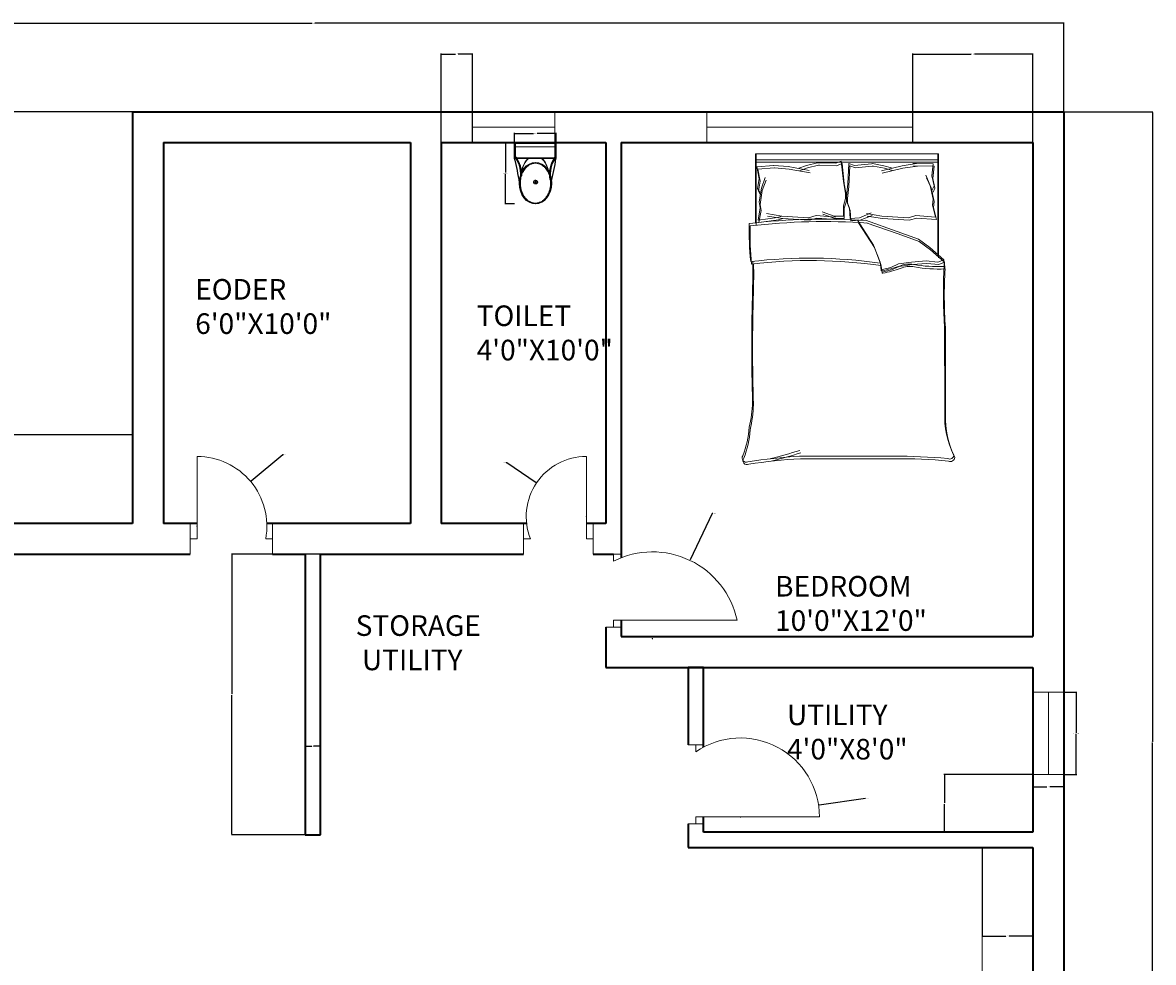
# Model space of a CAD drawing. Units: inches. Extents: x 2067 to 3463, y 1605 to 2723.
# Tile 5 of 10: x 2403 to 2733, y 1910 to 2184. Entities that reach past the tile are written whole.
import ezdxf

# ---------------------------------------------------------------- set-up
doc = ezdxf.new("R2010")
doc.units = ezdxf.units.IN
for name, color, linetype, lineweight in [('A-ANNO-DIMS', 2, 'Continuous', 18), ('A-AREA-IDEN', 7, 'Continuous', 18), ('A-DOOR', 3, 'Continuous', 18), ('A-FLOR-CASE', 8, 'Continuous', 18), ('A-FLOR-FIXT', 8, 'Continuous', 18), ('A-FURN', 8, 'Continuous', 13), ('A-GLAZ', 4, 'Continuous', 18), ('A-WALL', 7, 'Continuous', 35)]:
    doc.layers.add(name, color=color, linetype=linetype, lineweight=lineweight)
doc.styles.get("Standard").update_dxf_attribs({"font": 'arial.ttf'})
doc.dimstyles.get("Standard").update_dxf_attribs({"dimtxt": 0.18, "dimasz": 0.18, "dimexe": 0.18, "dimexo": 0.0625, "dimgap": 0.09, "dimtad": 0, "dimtih": 1, "dimtoh": 1, "dimdec": 4, "dimzin": 0, "dimdsep": 46, "dimtxsty": 'Standard', "dimcen": 0.09, "dimadec": 0, "dimazin": 0, "dimtfac": 1, "dimtdec": 4, "dimtofl": 0, "dimtmove": 0, "dimatfit": 3, "dimfxl": 1, "dimtolj": 1, "dimtzin": 0, "dimarcsym": 0})

# ---------------------------------------------------------------- blocks, each defined once
blk = doc.blocks.new('A$C31115884')
for p, q in [((283, 498), (223, 498)), ((258, 466), (258, 523)), ((0, 200), (0, 0)), ((520, 200), (0, 200)), ((10, 190), (10, 10)), ((510, 190), (10, 190)), ((510, 10), (510, 190)), ((520, 0), (520, 200)), ((510, 54), (0, 54)), ((10, 10), (510, 10)), ((0, 0), (520, 0))]:
    blk.add_line(p, q)
blk.add_circle((256, 496), 23.6)
for centre, radius, start, end in [((2778, -205), 2807, 165.4549, 171.7133), ((-295, 403), 365, 324.2091, 9.3499), ((-295, 403), 375, 324.2091, 9.3499), ((806, 403), 365, 170.6501, 215.7909), ((3237, 905), 2807, 188.2867, 194.5451), ((384, 406), 293, 190.2774, 224.1564), ((139, 406), 293, 315.8436, 2.6563), ((806, 403), 375, 179.2036, 215.7909)]:
    blk.add_arc(centre, radius, start, end)
blk.add_ellipse((256, 510), major_axis=(0, -261), ratio=0.772727)
blk.add_open_spline([(256, 259), (263, 259), (270, 260), (288, 262), (299, 265), (320, 273), (330, 278), (350, 291), (360, 299), (378, 316), (386, 326), (402, 347), (409, 358), (421, 383), (427, 395), (436, 422), (440, 436), (445, 465), (447, 480), (448, 509), (448, 524), (445, 553), (443, 568), (436, 596), (432, 610), (422, 636), (416, 649), (402, 672), (395, 683), (379, 703), (370, 712), (351, 728), (341, 735), (321, 746), (310, 751), (289, 757), (278, 759), (256, 761), (245, 761), (223, 757), (212, 754), (191, 746), (181, 741), (161, 728), (151, 720), (133, 703), (125, 693), (110, 672), (103, 660), (90, 636), (85, 623), (76, 596), (72, 582), (67, 553), (66, 538), (64, 509), (65, 494), (68, 465), (70, 450), (77, 422), (81, 408), (91, 382), (97, 370), (111, 346), (118, 335), (135, 316), (144, 307), (162, 291), (172, 284), (193, 273), (203, 269), (225, 262), (236, 260), (250, 259), (253, 259), (256, 259)], degree=3, knots=[0, 0, 0, 0, 0.110105, 0.110105, 0.285049, 0.285049, 0.459994, 0.459994, 0.634938, 0.634938, 0.809882, 0.809882, 0.984827, 0.984827, 1.159771, 1.159771, 1.334715, 1.334715, 1.50966, 1.50966, 1.684604, 1.684604, 1.859549, 1.859549, 2.034493, 2.034493, 2.209437, 2.209437, 2.384382, 2.384382, 2.559326, 2.559326, 2.73427, 2.73427, 2.909215, 2.909215, 3.084159, 3.084159, 3.259103, 3.259103, 3.434048, 3.434048, 3.608992, 3.608992, 3.783936, 3.783936, 3.958881, 3.958881, 4.133825, 4.133825, 4.30877, 4.30877, 4.483714, 4.483714, 4.658658, 4.658658, 4.833603, 4.833603, 5.008547, 5.008547, 5.183491, 5.183491, 5.358436, 5.358436, 5.53338, 5.53338, 5.708324, 5.708324, 5.883269, 5.883269, 6.058213, 6.058213, 6.233158, 6.233158, 6.283185, 6.283185, 6.283185, 6.283185])
blk = doc.blocks.new('BED-DOUBLE')
for p, q in [((3.86, 70.43), (3.86, 90.57)), ((3.86, 90.57), (57.01, 90.57)), ((4.12, 89.85), (4.12, 90.57)), ((4.12, 69.72), (4.12, 89.85)), ((57.01, 90.57), (57.01, 60.97)), ((57.01, 90.57), (57.26, 90.57)), ((57.26, 90.57), (57.26, 89.74)), ((57.26, 89.85), (57.26, 60.26)), ((3.86, 88.86), (57.01, 88.86)), ((4.12, 88.15), (57.26, 88.15)), ((4.33, 86.88), (4.97, 83.34)), ((4.34, 86.85), (9.1, 87.22)), ((4.59, 86.14), (9.35, 86.51)), ((4.59, 86.17), (5.23, 82.63)), ((9.1, 87.22), (9.21, 87.2)), ((9.21, 87.2), (13.46, 86.88)), ((9.35, 86.51), (9.47, 86.49)), ((9.47, 86.49), (13.72, 86.17)), ((13.46, 86.88), (19.57, 85.75)), ((13.72, 86.17), (19.83, 85.04)), ((16.52, 86.4), (18.77, 87.2)), ((16.77, 85.68), (19.02, 86.49)), ((18.77, 87.2), (21.98, 88)), ((19.02, 86.49), (22.24, 87.29)), ((21.98, 88), (22.34, 88)), ((22.24, 87.29), (22.6, 87.29)), ((22.34, 88), (27.29, 87.84)), ((22.6, 87.29), (27.54, 87.13)), ((27.29, 87.84), (28.89, 88.49)), ((27.54, 87.13), (29.15, 87.77)), ((28.89, 88.49), (29.54, 82.54)), ((29.15, 87.77), (29.79, 81.83)), ((31.11, 87.79), (30.84, 81.82)), ((31.36, 87.08), (31.09, 81.11)), ((32.76, 87.25), (31.11, 87.79)), ((33.01, 86.54), (31.36, 87.08)), ((37.68, 87.72), (32.76, 87.25)), ((37.93, 87.01), (33.01, 86.54)), ((38.04, 87.74), (37.68, 87.72)), ((38.29, 87.03), (37.93, 87.01)), ((41.29, 87.14), (38.04, 87.74)), ((41.55, 86.43), (38.29, 87.03)), ((46.61, 87.15), (40.58, 85.65)), ((46.86, 86.44), (40.84, 84.94)), ((43.59, 86.48), (41.29, 87.14)), ((43.85, 85.77), (41.55, 86.43)), ((50.83, 87.74), (46.61, 87.15)), ((51.09, 87.03), (46.86, 86.44)), ((55.73, 87.72), (49.72, 87.83)), ((49.72, 87.83), (50.83, 87.74)), ((55.98, 87.01), (49.97, 87.12)), ((49.97, 87.12), (51.09, 87.03)), ((55.73, 87.72), (55.3, 84.15)), ((55.98, 87.01), (55.56, 83.44)), ((4.97, 83.34), (4.49, 80.45)), ((5.23, 82.63), (4.75, 79.74)), ((5.62, 80.61), (6.74, 83.66)), ((5.87, 79.9), (7, 82.95)), ((29.54, 82.54), (30.18, 79)), ((54.83, 81.38), (53.52, 84.36)), ((55.09, 80.67), (53.77, 83.65)), ((55.3, 84.15), (55.97, 81.29)), ((55.56, 83.44), (56.22, 80.58)), ((4.49, 80.45), (5.13, 79.32)), ((4.75, 79.74), (5.39, 78.61)), ((4.97, 76.59), (5.62, 80.61)), ((5.23, 75.88), (5.87, 79.9)), ((29.79, 81.83), (30.43, 78.29)), ((30.84, 81.82), (30.42, 78.25)), ((31.09, 81.11), (30.67, 77.54)), ((55.73, 77.41), (54.83, 81.38)), ((55.98, 76.7), (55.09, 80.67)), ((55.97, 81.29), (55.39, 80.13)), ((56.22, 80.58), (55.65, 79.42)), ((5.3, 74.82), (4.97, 76.59)), ((5.55, 74.11), (5.23, 75.88)), ((30.18, 77.55), (29.54, 75.46)), ((30.43, 76.84), (29.79, 74.75)), ((30.18, 79), (30.18, 77.55)), ((30.42, 78.25), (30.51, 76.8)), ((30.43, 78.29), (30.43, 76.84)), ((30.51, 76.8), (31.28, 74.76)), ((30.67, 77.54), (30.76, 76.09)), ((30.76, 76.09), (31.54, 74.05)), ((55.51, 75.63), (55.73, 77.41)), ((55.77, 74.92), (55.98, 76.7)), ((4.65, 71.28), (5.3, 74.82)), ((4.91, 70.57), (5.55, 74.11)), ((7.1, 73.19), (11.58, 72.44)), ((19.38, 71.97), (21.56, 72.58)), ((21.56, 72.58), (27.26, 72.14)), ((26.8, 72.48), (23.31, 73.69)), ((27.06, 71.77), (23.56, 72.98)), ((29.54, 75.46), (29.54, 72.48)), ((29.79, 74.75), (29.79, 71.77)), ((31.28, 74.76), (31.47, 71.78)), ((31.54, 74.05), (31.72, 71.07)), ((34.19, 71.95), (37.61, 73.38)), ((34.45, 71.24), (37.86, 72.67)), ((36.21, 73.19), (40.7, 72.44)), ((48.49, 71.97), (50.67, 72.58)), ((50.67, 72.58), (56.38, 72.14)), ((56.38, 72.14), (55.51, 75.63)), ((56.63, 71.43), (55.77, 74.92)), ((10.32, 72.09), (4.65, 71.28)), ((10.57, 71.37), (4.91, 70.57)), ((7.35, 72.48), (11.83, 71.73)), ((11.58, 72.44), (10.32, 72.09)), ((11.83, 71.73), (10.57, 71.37)), ((11.58, 72.44), (19.38, 71.97)), ((11.83, 71.73), (19.63, 71.25)), ((19.63, 71.25), (21.81, 71.87)), ((21.81, 71.87), (27.52, 71.43)), ((29.54, 72.48), (26.8, 72.48)), ((29.79, 71.77), (27.06, 71.77)), ((31.47, 71.78), (34.19, 71.95)), ((31.72, 71.07), (34.45, 71.24)), ((33.65, 71.23), (38.31, 64.01)), ((33.9, 70.52), (38.56, 63.3)), ((45.2, 67.97), (35.92, 71.23)), ((45.45, 67.26), (36.18, 70.52)), ((36.47, 72.48), (40.95, 71.73)), ((40.7, 72.44), (48.49, 71.97)), ((40.95, 71.73), (48.74, 71.25)), ((48.74, 71.25), (50.92, 71.87)), ((50.92, 71.87), (56.63, 71.43)), ((51.4, 65.74), (45.2, 67.97)), ((51.65, 65.02), (45.45, 67.26)), ((38.31, 64.01), (40.2, 59.02)), ((38.56, 63.3), (40.46, 58.31)), ((54.67, 63.33), (51.4, 65.74)), ((54.92, 62.61), (51.65, 65.02)), ((58.79, 59.71), (54.67, 63.33)), ((49.33, 59.02), (53.64, 59.37)), ((53.64, 59.37), (57.08, 59.02)), ((59.04, 59), (54.92, 62.61)), ((57.08, 59.02), (58.79, 59.71)), ((58.88, 57.77), (58.79, 59.71, 4.3)), ((40.2, 59.02), (40.55, 56.79)), ((40.46, 58.31), (40.8, 56.07)), ((40.55, 56.79), (43.3, 57.47)), ((40.8, 56.07), (43.56, 56.76)), ((43.3, 57.47), (45.54, 58.51)), ((43.56, 56.76), (45.8, 57.8)), ((45.54, 58.51), (49.33, 59.02)), ((45.8, 57.8), (49.58, 58.31)), ((49.58, 58.31), (53.89, 58.66)), ((53.89, 58.66), (57.33, 58.31)), ((57.33, 58.31), (59.04, 59)), ((59.13, 57.06), (59.04, 59, 4.3)), ((16.75, 2.44), (44.12, 2.44)), ((17, 1.73), (44.38, 1.73))]:
    blk.add_line(p, q)
for centre, radius, start, end in [((94.7, 68.22), 92.64, 178.7218, 185.604), ((23.75, -111.88), 183.45, 86.0865, 96.7821), ((94.95, 67.51), 92.64, 178.7218, 185.604), ((24.01, -112.59), 183.45, 86.0865, 96.7821), ((19.74, -83.26), 143.47, 81.7845, 96.9006), ((20, -83.97), 143.47, 81.7845, 96.9006), ((-186.05, 55.9), 189.16, 358.4762, 1.0082), ((-185.79, 55.19), 189.16, 358.4762, 1.0082), ((40.74, 56.72), 0.205, 160.2464, 271.1377), ((34.64, 88.92), 32.98, 280.6617, 289.8806), ((40.99, 56.01), 0.205, 160.2464, 271.1377), ((34.9, 88.21), 32.98, 280.6617, 289.8806), ((48.64, 51.57), 6.92, 78.6608, 113.7384), ((48.9, 50.86), 6.92, 78.6608, 113.7384), ((57.08, 97.97), 40.24, 259.8763, 272.5657), ((57.33, 97.26), 40.24, 259.8763, 272.5657), ((202.68, 50.18), 144, 176.9791, 183.8365), ((202.94, 49.47), 144, 176.9791, 183.8365), ((539.13, 34.28), 536.33, 178.2277, 181.7185), ((539.38, 33.57), 536.33, 178.2277, 181.7185), ((-5013.77, 15.15), 5072.83, 0.00217, 0.28689), ((-5013.52, 14.44), 5072.83, 0.00217, 0.28689), ((-29.91, 18.82), 32.95, 346.0648, 358.9113), ((-29.66, 18.11), 32.95, 346.0648, 358.9113), ((84.69, 14.21), 25.65, 177.4714, 206.4681), ((84.94, 13.5), 25.65, 177.4714, 206.4681), ((-24.09, 12.42), 26.2, 337.9751, 356.652), ((-23.83, 11.71), 26.2, 337.9751, 356.652), ((-19.15, 116.93), 118.38, 283.3832, 287.7053), ((-18.9, 116.22), 118.38, 283.3832, 287.7053), ((1.21, 1.92), 1.21, 146.1736, 293.4781), ((1.46, 1.21), 1.21, 146.1736, 293.4781), ((23.83, -132.77), 135.4, 92.9958, 99.4091), ((24.08, -133.48), 135.4, 92.9958, 99.4091), ((45.76, -145.49), 147.94, 84.4998, 90.6351), ((46.02, -146.2), 147.94, 84.4998, 90.6351), ((60.5, 2.86), 1.23, 242.6588, 356.02), ((60.76, 2.15), 1.23, 242.6588, 356.02)]:
    blk.add_arc(centre, radius, start, end)
blk = doc.blocks.new('WIN-PLAN-24-OFFSET')
for p, q in [((0, 24), (9, 24)), ((9, 24), (4.5, 24)), ((4.5, 24), (4.5, 0)), ((4.5, 0), (0, 0)), ((0, 0), (9, 0))]:
    blk.add_line(p, q)
blk = doc.blocks.new('WIN-PLAN-24-ALIGNED')
for p, q in [((0, 0), (0, 9)), ((0, 9), (0, 4.5)), ((24, 4.5), (24, 9)), ((24, 9), (24, 0)), ((0, 4.5), (24, 4.5))]:
    blk.add_line(p, q)
blk = doc.blocks.new('WIN-PLAN-60-ALIGNED')
for p, q in [((0, 0), (0, 9)), ((0, 9), (0, 4.5)), ((60, 4.5), (60, 9)), ((60, 9), (60, 0)), ((0, 4.5), (60, 4.5))]:
    blk.add_line(p, q)
blk = doc.blocks.new('*D14')
at = {"layer": 'A-ANNO-DIMS', "color": 0, "lineweight": -2, "transparency": 16777216}
for p, q in [((2546.29, 2149.23), (2543.49, 2149.23)), ((2543.67, 2149.05), (2543.67, 2140.48)), ((2543.67, 2131.54), (2543.67, 2140.11)), ((2546.29, 2131.36), (2543.49, 2131.36))]:
    blk.add_line(p, q, dxfattribs=at)
at = {"layer": 'A-ANNO-DIMS', "color": 0, "transparency": 16777216}
for points in [[(2543.64, 2149.05), (2543.7, 2149.05), (2543.67, 2149.23)], [(2543.64, 2131.54), (2543.7, 2131.54), (2543.67, 2131.36)]]:
    blk.add_solid(points, dxfattribs=at)
at = {"layer": 'Defpoints', "color": 0, "transparency": 16777216}
for p in [(2546.35, 2149.23), (2543.67, 2131.36), (2546.35, 2131.36)]:
    blk.add_point(p, dxfattribs=at)
at = {"layer": 'A-ANNO-DIMS', "color": 0, "transparency": 16777216, "insert": (2543.67, 2140.3), "char_height": 0.18, "attachment_point": 5}
blk.add_mtext('\\A1;WC 18 TYP.', dxfattribs=at)
blk = doc.blocks.new('*D15')
at = {"layer": 'A-ANNO-DIMS', "color": 0, "lineweight": -2, "transparency": 16777216}
for p, q in [((2546.35, 2149.29), (2546.35, 2152.09)), ((2546.53, 2151.91), (2551.86, 2151.91)), ((2558.23, 2151.91), (2552.9, 2151.91)), ((2558.41, 2149.29), (2558.41, 2152.09))]:
    blk.add_line(p, q, dxfattribs=at)
at = {"layer": 'A-ANNO-DIMS', "color": 0, "transparency": 16777216}
for points in [[(2546.53, 2151.94), (2546.53, 2151.88), (2546.35, 2151.91)], [(2558.23, 2151.94), (2558.23, 2151.88), (2558.41, 2151.91)]]:
    blk.add_solid(points, dxfattribs=at)
at = {"layer": 'Defpoints', "color": 0, "transparency": 16777216}
for p in [(2546.35, 2151.91), (2546.35, 2149.23), (2558.41, 2149.23)]:
    blk.add_point(p, dxfattribs=at)
at = {"layer": 'A-ANNO-DIMS', "color": 0, "transparency": 16777216, "insert": (2552.38, 2151.91), "char_height": 0.18, "attachment_point": 5}
blk.add_mtext('\\A1;12 TYP.', dxfattribs=at)
blk = doc.blocks.new('*D18')
at = {"layer": 'A-ANNO-DIMS', "color": 0, "lineweight": -2, "transparency": 16777216}
for p, q in [((2706.51, 1989), (2710.23, 1989)), ((2710.05, 1988.82), (2710.05, 1977.18)), ((2710.05, 1965.18), (2710.05, 1976.82)), ((2706.51, 1965), (2710.23, 1965))]:
    blk.add_line(p, q, dxfattribs=at)
at = {"layer": 'A-ANNO-DIMS', "color": 0, "transparency": 16777216}
for points in [[(2710.02, 1988.82), (2710.08, 1988.82), (2710.05, 1989)], [(2710.02, 1965.18), (2710.08, 1965.18), (2710.05, 1965)]]:
    blk.add_solid(points, dxfattribs=at)
at = {"layer": 'Defpoints', "color": 0, "transparency": 16777216}
for p in [(2706.45, 1989), (2710.05, 1989), (2706.45, 1965)]:
    blk.add_point(p, dxfattribs=at)
at = {"layer": 'A-ANNO-DIMS', "color": 0, "transparency": 16777216, "insert": (2710.05, 1977), "char_height": 0.18, "attachment_point": 5}
blk.add_mtext('\\A1;WINDOW 24 TYP.', dxfattribs=at)
blk = doc.blocks.new('*D19')
at = {"layer": 'A-ANNO-DIMS', "color": 0, "lineweight": -2, "transparency": 16777216}
for p, q in [((2697.45, 1964.94), (2697.45, 1961.22)), ((2706.45, 1964.94), (2706.45, 1961.22)), ((2697.63, 1961.4), (2701.49, 1961.4)), ((2706.27, 1961.4), (2702.41, 1961.4))]:
    blk.add_line(p, q, dxfattribs=at)
at = {"layer": 'A-ANNO-DIMS', "color": 0, "transparency": 16777216}
for points in [[(2697.63, 1961.43), (2697.63, 1961.37), (2697.45, 1961.4)], [(2706.27, 1961.43), (2706.27, 1961.37), (2706.45, 1961.4)]]:
    blk.add_solid(points, dxfattribs=at)
at = {"layer": 'Defpoints', "color": 0, "transparency": 16777216}
for p in [(2697.45, 1965), (2706.45, 1965), (2706.45, 1961.4)]:
    blk.add_point(p, dxfattribs=at)
at = {"layer": 'A-ANNO-DIMS', "color": 0, "transparency": 16777216, "insert": (2701.95, 1961.4), "char_height": 0.18, "attachment_point": 5}
blk.add_mtext('\\A1;9 TYP.', dxfattribs=at)
blk = doc.blocks.new('*D28')
at = {"layer": 'A-ANNO-DIMS', "color": 0, "lineweight": -2, "transparency": 16777216}
for p, q in [((2268.95, 2038.28), (2268.95, 2184.21)), ((2269.13, 2184.03), (2487.3, 2184.03)), ((2706.27, 2184.03), (2488.1, 2184.03)), ((2706.45, 2158.29), (2706.45, 2184.21))]:
    blk.add_line(p, q, dxfattribs=at)
at = {"layer": 'A-ANNO-DIMS', "color": 0, "transparency": 16777216}
for points in [[(2269.13, 2184.06), (2269.13, 2184), (2268.95, 2184.03)], [(2706.27, 2184.06), (2706.27, 2184), (2706.45, 2184.03)]]:
    blk.add_solid(points, dxfattribs=at)
at = {"layer": 'Defpoints', "color": 0, "transparency": 16777216}
for p in [(2706.45, 2184.03), (2706.45, 2158.23), (2268.95, 2038.22)]:
    blk.add_point(p, dxfattribs=at)
at = {"layer": 'A-ANNO-DIMS', "color": 0, "transparency": 16777216, "insert": (2487.7, 2184.03), "char_height": 0.18, "attachment_point": 5}
blk.add_mtext('\\A1;437.5', dxfattribs=at)
blk = doc.blocks.new('*D29')
at = {"layer": 'A-ANNO-DIMS', "color": 0, "lineweight": -2, "transparency": 16777216}
for p, q in [((2706.51, 2158.23), (2732.43, 2158.23)), ((2732.25, 2158.05), (2732.25, 1974.66)), ((2732.25, 1790.91), (2732.25, 1974.3)), ((2706.51, 1790.73), (2732.43, 1790.73))]:
    blk.add_line(p, q, dxfattribs=at)
at = {"layer": 'A-ANNO-DIMS', "color": 0, "transparency": 16777216}
for points in [[(2732.22, 2158.05), (2732.28, 2158.05), (2732.25, 2158.23)], [(2732.22, 1790.91), (2732.28, 1790.91), (2732.25, 1790.73)]]:
    blk.add_solid(points, dxfattribs=at)
at = {"layer": 'Defpoints', "color": 0, "transparency": 16777216}
for p in [(2706.45, 2158.23), (2732.25, 2158.23), (2706.45, 1790.73)]:
    blk.add_point(p, dxfattribs=at)
at = {"layer": 'A-ANNO-DIMS', "color": 0, "transparency": 16777216, "insert": (2732.25, 1974.48), "char_height": 0.18, "attachment_point": 5}
blk.add_mtext('\\A1;367.5', dxfattribs=at)
blk = doc.blocks.new('*D30')
at = {"layer": 'A-ANNO-DIMS', "color": 0, "lineweight": -2, "transparency": 16777216}
for p, q in [((2268.95, 2038.28), (2268.95, 2064.2)), ((2269.13, 2064.02), (2351.67, 2064.02)), ((2434.77, 2064.02), (2352.23, 2064.02)), ((2434.95, 2038.28), (2434.95, 2064.2))]:
    blk.add_line(p, q, dxfattribs=at)
at = {"layer": 'A-ANNO-DIMS', "color": 0, "transparency": 16777216}
for points in [[(2269.13, 2064.05), (2269.13, 2063.99), (2268.95, 2064.02)], [(2434.77, 2064.05), (2434.77, 2063.99), (2434.95, 2064.02)]]:
    blk.add_solid(points, dxfattribs=at)
at = {"layer": 'Defpoints', "color": 0, "transparency": 16777216}
for p in [(2434.95, 2064.02), (2268.95, 2038.22), (2434.95, 2038.22)]:
    blk.add_point(p, dxfattribs=at)
at = {"layer": 'A-ANNO-DIMS', "color": 0, "transparency": 16777216, "insert": (2351.95, 2064.02), "char_height": 0.18, "attachment_point": 5}
blk.add_mtext('\\A1;166', dxfattribs=at)
blk = doc.blocks.new('*D31')
at = {"layer": 'A-ANNO-DIMS', "color": 0, "lineweight": -2, "transparency": 16777216}
for p, q in [((2434.89, 2158.23), (2242.97, 2158.23)), ((2243.15, 2158.05), (2243.15, 2098.41)), ((2243.15, 2038.4), (2243.15, 2098.04)), ((2434.89, 2038.22), (2242.97, 2038.22))]:
    blk.add_line(p, q, dxfattribs=at)
at = {"layer": 'A-ANNO-DIMS', "color": 0, "transparency": 16777216}
for points in [[(2243.12, 2158.05), (2243.18, 2158.05), (2243.15, 2158.23)], [(2243.12, 2038.4), (2243.18, 2038.4), (2243.15, 2038.22)]]:
    blk.add_solid(points, dxfattribs=at)
at = {"layer": 'Defpoints', "color": 0, "transparency": 16777216}
for p in [(2243.15, 2158.23), (2434.95, 2158.23), (2434.95, 2038.22)]:
    blk.add_point(p, dxfattribs=at)
at = {"layer": 'A-ANNO-DIMS', "color": 0, "transparency": 16777216, "insert": (2243.15, 2098.22), "char_height": 0.18, "attachment_point": 5}
blk.add_mtext('\\A1;120.01', dxfattribs=at)
blk = doc.blocks.new('*D44')
at = {"layer": 'A-ANNO-DIMS', "color": 0, "lineweight": -2, "transparency": 16777216}
for p, q in [((2697.39, 1965), (2671.47, 1965)), ((2671.65, 1964.82), (2671.65, 1956.8)), ((2671.65, 1948.41), (2671.65, 1956.43)), ((2697.39, 1948.23), (2671.47, 1948.23))]:
    blk.add_line(p, q, dxfattribs=at)
at = {"layer": 'A-ANNO-DIMS', "color": 0, "transparency": 16777216}
for points in [[(2671.62, 1964.82), (2671.68, 1964.82), (2671.65, 1965)], [(2671.62, 1948.41), (2671.68, 1948.41), (2671.65, 1948.23)]]:
    blk.add_solid(points, dxfattribs=at)
at = {"layer": 'Defpoints', "color": 0, "transparency": 16777216}
for p in [(2671.65, 1965), (2697.45, 1965), (2697.45, 1948.23)]:
    blk.add_point(p, dxfattribs=at)
at = {"layer": 'A-ANNO-DIMS', "color": 0, "transparency": 16777216, "insert": (2671.65, 1956.62), "char_height": 0.18, "attachment_point": 5}
blk.add_mtext('\\A1;16.77', dxfattribs=at)
blk = doc.blocks.new('*D45')
at = {"layer": 'A-ANNO-DIMS', "color": 0, "lineweight": -2, "transparency": 16777216}
for p, q in [((2662.42, 2149.29), (2662.42, 2175.21)), ((2662.6, 2175.03), (2679.47, 2175.03)), ((2697.27, 2175.03), (2680.4, 2175.03)), ((2697.45, 2149.29), (2697.45, 2175.21))]:
    blk.add_line(p, q, dxfattribs=at)
at = {"layer": 'A-ANNO-DIMS', "color": 0, "transparency": 16777216}
for points in [[(2662.6, 2175.06), (2662.6, 2175), (2662.42, 2175.03)], [(2697.27, 2175.06), (2697.27, 2175), (2697.45, 2175.03)]]:
    blk.add_solid(points, dxfattribs=at)
at = {"layer": 'Defpoints', "color": 0, "transparency": 16777216}
for p in [(2697.45, 2175.03), (2662.42, 2149.23), (2697.45, 2149.23)]:
    blk.add_point(p, dxfattribs=at)
at = {"layer": 'A-ANNO-DIMS', "color": 0, "transparency": 16777216, "insert": (2679.94, 2175.03), "char_height": 0.18, "attachment_point": 5}
blk.add_mtext('\\A1;35.024', dxfattribs=at)
blk = doc.blocks.new('*D46')
at = {"layer": 'A-ANNO-DIMS', "color": 0, "lineweight": -2, "transparency": 16777216}
for p, q in [((2524.95, 2149.29), (2524.95, 2175.21)), ((2525.13, 2175.03), (2529.12, 2175.03)), ((2533.89, 2175.03), (2529.9, 2175.03)), ((2534.07, 2149.29), (2534.07, 2175.21))]:
    blk.add_line(p, q, dxfattribs=at)
at = {"layer": 'A-ANNO-DIMS', "color": 0, "transparency": 16777216}
for points in [[(2525.13, 2175.06), (2525.13, 2175), (2524.95, 2175.03)], [(2533.89, 2175.06), (2533.89, 2175), (2534.07, 2175.03)]]:
    blk.add_solid(points, dxfattribs=at)
at = {"layer": 'Defpoints', "color": 0, "transparency": 16777216}
for p in [(2534.07, 2175.03), (2524.95, 2149.23), (2534.07, 2149.23)]:
    blk.add_point(p, dxfattribs=at)
at = {"layer": 'A-ANNO-DIMS', "color": 0, "transparency": 16777216, "insert": (2529.51, 2175.03), "char_height": 0.18, "attachment_point": 5}
blk.add_mtext('\\A1;9.127', dxfattribs=at)
blk = doc.blocks.new('*D47')
at = {"layer": 'A-ANNO-DIMS', "color": 0, "lineweight": -2, "transparency": 16777216}
for p, q in [((2489.67, 2029.23), (2463.76, 2029.23)), ((2463.94, 2029.05), (2463.94, 1988.54)), ((2463.94, 1947.67), (2463.94, 1988.18)), ((2489.67, 1947.49), (2463.76, 1947.49))]:
    blk.add_line(p, q, dxfattribs=at)
at = {"layer": 'A-ANNO-DIMS', "color": 0, "transparency": 16777216}
for points in [[(2463.91, 2029.05), (2463.97, 2029.05), (2463.94, 2029.23)], [(2463.91, 1947.67), (2463.97, 1947.67), (2463.94, 1947.49)]]:
    blk.add_solid(points, dxfattribs=at)
at = {"layer": 'Defpoints', "color": 0, "transparency": 16777216}
for p in [(2463.94, 2029.23), (2489.74, 2029.23), (2489.74, 1947.49)]:
    blk.add_point(p, dxfattribs=at)
at = {"layer": 'A-ANNO-DIMS', "color": 0, "transparency": 16777216, "insert": (2463.94, 1988.36), "char_height": 0.18, "attachment_point": 5}
blk.add_mtext('\\A1;81.74', dxfattribs=at)
blk = doc.blocks.new('*D48')
at = {"layer": 'A-ANNO-DIMS', "color": 0, "lineweight": -2, "transparency": 16777216}
for p, q in [((2485.24, 1947.55), (2485.24, 1973.47)), ((2485.42, 1973.29), (2487.23, 1973.29)), ((2489.56, 1973.29), (2487.74, 1973.29)), ((2489.74, 1947.55), (2489.74, 1973.47))]:
    blk.add_line(p, q, dxfattribs=at)
at = {"layer": 'A-ANNO-DIMS', "color": 0, "transparency": 16777216}
for points in [[(2485.42, 1973.32), (2485.42, 1973.26), (2485.24, 1973.29)], [(2489.56, 1973.32), (2489.56, 1973.26), (2489.74, 1973.29)]]:
    blk.add_solid(points, dxfattribs=at)
at = {"layer": 'Defpoints', "color": 0, "transparency": 16777216}
for p in [(2489.74, 1973.29), (2485.24, 1947.49), (2489.74, 1947.49)]:
    blk.add_point(p, dxfattribs=at)
at = {"layer": 'A-ANNO-DIMS', "color": 0, "transparency": 16777216, "insert": (2487.49, 1973.29), "char_height": 0.18, "attachment_point": 5}
blk.add_mtext('\\A1;4.5', dxfattribs=at)
blk = doc.blocks.new('*D49')
at = {"layer": 'A-ANNO-DIMS', "color": 0, "lineweight": -2, "transparency": 16777216}
for p, q in [((2682.6, 1943.67), (2682.6, 1917.75)), ((2697.45, 1943.67), (2697.45, 1917.75)), ((2682.78, 1917.93), (2689.57, 1917.93)), ((2697.27, 1917.93), (2690.48, 1917.93))]:
    blk.add_line(p, q, dxfattribs=at)
at = {"layer": 'A-ANNO-DIMS', "color": 0, "transparency": 16777216}
for points in [[(2682.78, 1917.96), (2682.78, 1917.9), (2682.6, 1917.93)], [(2697.27, 1917.96), (2697.27, 1917.9), (2697.45, 1917.93)]]:
    blk.add_solid(points, dxfattribs=at)
at = {"layer": 'Defpoints', "color": 0, "transparency": 16777216}
for p in [(2682.6, 1943.73), (2697.45, 1943.73), (2682.6, 1917.93)]:
    blk.add_point(p, dxfattribs=at)
at = {"layer": 'A-ANNO-DIMS', "color": 0, "transparency": 16777216, "insert": (2690.02, 1917.93), "char_height": 0.18, "attachment_point": 5}
blk.add_mtext('\\A1;14.852', dxfattribs=at)
blk = doc.blocks.new('*D103')
at = {"layer": 'A-ANNO-DIMS', "color": 0, "lineweight": -2, "transparency": 16777216}
for p, q in [((2603.97, 2041.09), (2597.51, 2027.61)), ((2604.15, 2041.09), (2603.97, 2041.09)), ((2586.45, 2004.72), (2586.63, 2004.72)), ((2586.54, 2004.63), (2586.54, 2004.81))]:
    blk.add_line(p, q, dxfattribs=at)
at = {"layer": 'A-ANNO-DIMS', "color": 0, "transparency": 16777216}
blk.add_solid([(2597.49, 2027.63), (2597.54, 2027.6), (2597.44, 2027.45)], dxfattribs=at)
at = {"layer": 'Defpoints', "color": 0, "transparency": 16777216}
for p in [(2597.44, 2027.45), (2586.54, 2004.72)]:
    blk.add_point(p, dxfattribs=at)
at = {"layer": 'A-ANNO-DIMS', "color": 0, "transparency": 16777216, "insert": (2604.62, 2041.09), "char_height": 0.18, "attachment_point": 5}
blk.add_mtext('\\A1;R25.21', dxfattribs=at)
blk = doc.blocks.new('*D104')
at = {"layer": 'A-ANNO-DIMS', "color": 0, "lineweight": -2, "transparency": 16777216}
for p, q in [((2648.61, 1958.03), (2635.13, 1956.05)), ((2612.1, 1952.68), (2612.28, 1952.68)), ((2612.19, 1952.59), (2612.19, 1952.77))]:
    blk.add_line(p, q, dxfattribs=at)
at = {"layer": 'A-ANNO-DIMS', "color": 0, "transparency": 16777216}
blk.add_solid([(2635.13, 1956.08), (2635.14, 1956.02), (2634.95, 1956.02)], dxfattribs=at)
at = {"layer": 'Defpoints', "color": 0, "transparency": 16777216}
for p in [(2634.95, 1956.02), (2612.19, 1952.68)]:
    blk.add_point(p, dxfattribs=at)
at = {"layer": 'A-ANNO-DIMS', "color": 0, "transparency": 16777216, "insert": (2649.16, 1958.03), "char_height": 0.18, "attachment_point": 5}
blk.add_mtext('\\A1;R23.003', dxfattribs=at)
blk = doc.blocks.new('*D105')
at = {"layer": 'A-ANNO-DIMS', "color": 0, "lineweight": -2, "transparency": 16777216}
for p, q in [((2478.79, 2058.22), (2469.56, 2050.53)), ((2478.97, 2058.22), (2478.79, 2058.22)), ((2453.71, 2037.41), (2453.89, 2037.41)), ((2453.8, 2037.32), (2453.8, 2037.5))]:
    blk.add_line(p, q, dxfattribs=at)
at = {"layer": 'A-ANNO-DIMS', "color": 0, "transparency": 16777216}
blk.add_solid([(2469.54, 2050.55), (2469.57, 2050.51), (2469.42, 2050.41)], dxfattribs=at)
at = {"layer": 'Defpoints', "color": 0, "transparency": 16777216}
for p in [(2469.42, 2050.41), (2453.8, 2037.41)]:
    blk.add_point(p, dxfattribs=at)
at = {"layer": 'A-ANNO-DIMS', "color": 0, "transparency": 16777216, "insert": (2479.45, 2058.22), "char_height": 0.18, "attachment_point": 5}
blk.add_mtext('\\A1;R20.32', dxfattribs=at)
blk = doc.blocks.new('*D106')
at = {"layer": 'A-ANNO-DIMS', "color": 0, "lineweight": -2, "transparency": 16777216}
for p, q in [((2543.86, 2055.96), (2544.04, 2055.96)), ((2544.04, 2055.96), (2552.59, 2050.15)), ((2567.16, 2040.19), (2567.34, 2040.19)), ((2567.25, 2040.1), (2567.25, 2040.28))]:
    blk.add_line(p, q, dxfattribs=at)
at = {"layer": 'A-ANNO-DIMS', "color": 0, "transparency": 16777216}
blk.add_solid([(2552.61, 2050.17), (2552.58, 2050.12), (2552.74, 2050.05)], dxfattribs=at)
at = {"layer": 'Defpoints', "color": 0, "transparency": 16777216}
for p in [(2552.74, 2050.05), (2567.25, 2040.19)]:
    blk.add_point(p, dxfattribs=at)
at = {"layer": 'A-ANNO-DIMS', "color": 0, "transparency": 16777216, "insert": (2543.31, 2055.96), "char_height": 0.18, "attachment_point": 5}
blk.add_mtext('\\A1;R17.537', dxfattribs=at)

msp = doc.modelspace()

# ---------------------------------------------------------------- linework, layer by layer
at = {"layer": 'A-DOOR'}
for p, q in [((2453.8016, 2033.7309), (2453.8016, 2057.7309)), ((2567.2496, 2033.7309), (2567.2496, 2057.7309)), ((2451.8016, 2038.2309), (2451.8016, 2029.2171)), ((2475.7865, 2038.2309), (2475.7865, 2029.2171)), ((2548.9477, 2038.2309), (2548.9477, 2029.2171)), ((2548.9477, 2029.2309), (2548.9477, 2038.2309)), ((2569.2496, 2038.2309), (2569.2496, 2029.2171)), ((2451.8016, 2029.2171), (2451.8016, 2033.7309)), ((2451.8016, 2033.7309), (2453.8016, 2033.7309)), ((2475.7865, 2033.7309), (2473.7865, 2033.7309)), ((2475.7865, 2029.2171), (2475.7865, 2033.7309)), ((2548.9477, 2033.7309), (2550.9477, 2033.7309)), ((2569.2496, 2033.7309), (2567.2496, 2033.7309)), ((2569.2496, 2029.2171), (2569.2496, 2033.7309)), ((2572.9477, 2029.2309), (2577.4477, 2029.2309)), ((2577.4477, 2029.2309), (2575.1977, 2029.2309)), ((2575.1977, 2029.2309), (2575.1977, 2027.2309)), ((2572.9477, 2007.9806), (2577.4477, 2007.9806)), ((2575.1977, 2007.9806), (2575.1977, 2009.9806)), ((2575.1977, 2009.9806), (2611.1977, 2009.9806)), ((2577.4477, 2007.9806), (2575.1977, 2007.9806)), ((2601.4477, 1973.6564), (2596.9477, 1973.6564)), ((2596.9477, 1973.6564), (2599.1977, 1973.6564)), ((2599.1977, 1973.6564), (2599.1977, 1971.6564)), ((2599.1977, 1950.6775), (2599.1977, 1952.6775)), ((2599.1977, 1952.6775), (2635.1977, 1952.6775)), ((2601.4477, 1950.6775), (2596.9477, 1950.6775)), ((2596.9477, 1950.6775), (2599.1977, 1950.6775))]:
    msp.add_line(p, q, dxfattribs=at)
for centre, radius, start, end in [((2453.8016, 2037.4101), 20.3207, 349.568455, 90), ((2567.2496, 2040.1943), 17.5365, 90, 201.627628), ((2586.5426, 2004.7172), 25.2106, 12.050733, 116.744146), ((2612.1949, 1952.6775), 23.0028, 0, 124.404259)]:
    msp.add_arc(centre, radius, start, end, dxfattribs=at)
at = {"layer": 'A-FLOR-CASE'}
msp.add_line((2682.5961, 1811.0125), (2682.5961, 1943.7309), dxfattribs=at)
at = {"layer": 'A-GLAZ'}
msp.add_line((2662.4234, 2158.2309), (2662.4234, 2158.2309), dxfattribs=at)
at = {"layer": 'A-WALL'}
for p, q in [((2434.9477, 2158.2309), (2706.4477, 2158.2309)), ((2434.9477, 2158.2309), (2434.9477, 2038.2171)), ((2706.4477, 2158.2309), (2706.4477, 1790.7309)), ((2443.9477, 2149.2309), (2515.9477, 2149.2309)), ((2443.9477, 2149.2309), (2443.9477, 2038.2309)), ((2443.9477, 2149.2309), (2443.9477, 2038.2309)), ((2515.9477, 2149.2309), (2515.9477, 2038.2309)), ((2524.9477, 2149.2309), (2524.9477, 2038.2309)), ((2524.9477, 2149.2309), (2572.9477, 2149.2309)), ((2572.9477, 2149.2309), (2572.9477, 2038.2309)), ((2577.4477, 2149.2309), (2577.4477, 2028.2301)), ((2577.4477, 2149.2309), (2697.4477, 2149.2309)), ((2697.4477, 2149.2309), (2697.4477, 2005.2309)), ((2434.9477, 2038.2171), (2268.9477, 2038.2171)), ((2453.8016, 2038.2309), (2443.9477, 2038.2309)), ((2515.9477, 2038.2309), (2474.1057, 2038.2309)), ((2549.8233, 2038.2309), (2524.9477, 2038.2309)), ((2572.9477, 2038.2309), (2567.2496, 2038.2309)), ((2277.9477, 2029.2171), (2451.8016, 2029.2171)), ((2443.9477, 2029.2309), (2451.8016, 2029.2309)), ((2475.7865, 2029.2309), (2485.2361, 2029.2309)), ((2485.2361, 2029.2309), (2485.2361, 1947.4908)), ((2489.7361, 1947.4908), (2489.7361, 2029.2309)), ((2489.7361, 2029.2309), (2548.9477, 2029.2309)), ((2569.2496, 2029.2309), (2572.9477, 2029.2309)), ((2569.2496, 2029.2171), (2575.1977, 2029.2171)), ((2572.9477, 2007.9806), (2572.9477, 1996.2309)), ((2577.4477, 2009.9806), (2577.4477, 2005.2309)), ((2577.4477, 2005.2309), (2697.4477, 2005.2309)), ((2572.9477, 1996.2309), (2697.4477, 1996.2309)), ((2596.9477, 1996.2309), (2596.9477, 1973.6564)), ((2601.4477, 1996.2309), (2596.9477, 1996.2309)), ((2596.9477, 1996.2309), (2596.9477, 1973.6564)), ((2601.4477, 1973.0153), (2601.4477, 1996.2309)), ((2601.4477, 1973.0153), (2601.4477, 1996.2309)), ((2625.4477, 1996.2309), (2697.4477, 1996.2309)), ((2697.4477, 1996.2309), (2697.4477, 1948.2309)), ((2601.4477, 1948.2309), (2601.4477, 1952.6775)), ((2601.4477, 1948.2309), (2601.4477, 1952.6775)), ((2596.9477, 1950.6775), (2596.9477, 1948.2309)), ((2596.9477, 1950.6775), (2596.9477, 1943.7309)), ((2596.9477, 1948.2309), (2596.9477, 1943.7309)), ((2697.4477, 1948.2309), (2601.4477, 1948.2309)), ((2485.2361, 1947.4908), (2489.7361, 1947.4908)), ((2596.9477, 1943.7309), (2697.4477, 1943.7309)), ((2697.4477, 1943.7309), (2697.4477, 1799.7309))]:
    msp.add_line(p, q, dxfattribs=at)

# ---------------------------------------------------------------- block references
at = {"layer": 'A-FLOR-FIXT', "xscale": 0.0231892354596934, "yscale": 0.0231892354596934, "zscale": 0.0231892354596934, "rotation": 180}
for p in [(2558.3068, 2149.2309), (2558.4074, 2149.2309)]:
    msp.add_blockref('A$C31115884', p, dxfattribs=at)
at = {"layer": 'A-FURN'}
msp.add_blockref('BED-DOUBLE', (2612.667, 2055.357), dxfattribs=at)
at = {"layer": 'A-GLAZ'}
for name, p in [('WIN-PLAN-24-ALIGNED', (2534.075, 2149.231)), ('WIN-PLAN-60-ALIGNED', (2602.423, 2149.231)), ('WIN-PLAN-24-OFFSET', (2697.448, 1965))]:
    msp.add_blockref(name, p, dxfattribs=at)

# ---------------------------------------------------------------- texts
at = {"layer": 'A-AREA-IDEN', "char_height": 6, "attachment_point": 1}
for s, width, insert in [('EODER\\P6\'0"X10\'0"', 193.981676, (2453.2274, 2109.4618)), ('TOILET\\P4\'0"X10\'0"', 128.293511, (2535.2783, 2101.7579)), ('BEDROOM\\P10\'0"X12\'0"', 113.54788, (2622.2658, 2022.9086)), ('STORAGE\\P UTILITY', 67.677502, (2500.0015, 2011.4414)), ('UTILITY\\P4\'0"X8\'0"', 59.723087, (2625.7411, 1985.4168))]:
    msp.add_mtext_dynamic_manual_height_columns(s, width=width, gutter_width=12.5, heights=[0], dxfattribs=dict(at, insert=insert))

# ---------------------------------------------------------------- dimensions: what is measured, and where the dimension line sits
at = {"layer": 'A-ANNO-DIMS'}
for base, p1, p2, override, picture, middle in [((2706.4477, 2184.0309), (2268.9477, 2038.2171), (2706.4477, 2158.2309), {"dimdec": 1, "dimlfac": 1, "dimrnd": 0, "dimzin": 0, "dimdsep": 46, "dimlunit": 2}, '*D28', (2487.6977, 2184.0309)), ((2534.0749, 2175.0309), (2524.9477, 2149.2309), (2534.0749, 2149.2309), {"dimdec": 3, "dimlfac": 1, "dimrnd": 0, "dimzin": 0, "dimdsep": 46, "dimlunit": 2}, '*D46', (2529.5113, 2175.0309)), ((2697.4477, 2175.0309), (2662.4234, 2149.2309), (2697.4477, 2149.2309), {"dimdec": 3, "dimlfac": 1, "dimrnd": 0, "dimzin": 0, "dimdsep": 46, "dimlunit": 2}, '*D45', (2679.9355, 2175.0309)), ((2434.9477, 2064.0171), (2268.9477, 2038.2171), (2434.9477, 2038.2171), {"dimdec": 0, "dimlfac": 1, "dimrnd": 0, "dimzin": 0, "dimdsep": 46, "dimlunit": 2}, '*D30', (2351.9477, 2064.0171)), ((2489.7361, 1973.2908), (2485.2361, 1947.4908), (2489.7361, 1947.4908), {"dimdec": 1, "dimlfac": 1, "dimrnd": 0, "dimzin": 0, "dimdsep": 46, "dimlunit": 2}, '*D48', (2487.4861, 1973.2908))]:
    dim = msp.add_linear_dim(base=base, p1=p1, p2=p2, dimstyle='Standard', override=override, dxfattribs=at)
    dim.commit()
    dim.dimension.update_dxf_attribs({"geometry": picture, "text_midpoint": middle})
for base, p1, p2, angle, override, picture, middle in [((2243.1477, 2158.2309), (2434.9477, 2038.2171), (2434.9477, 2158.2309), 90, {"dimdec": 2, "dimlfac": 1, "dimrnd": 0, "dimzin": 0, "dimdsep": 46, "dimlunit": 2}, '*D31', (2243.1477, 2098.224)), ((2732.2477, 2158.2309), (2706.4477, 1790.7309), (2706.4477, 2158.2309), 90, {"dimdec": 1, "dimlfac": 1, "dimrnd": 0, "dimzin": 0, "dimdsep": 46, "dimlunit": 2}, '*D29', (2732.2477, 1974.4809)), ((2463.9361, 2029.2309), (2489.7361, 1947.4908), (2489.7361, 2029.2309), 90, {"dimdec": 2, "dimlfac": 1, "dimrnd": 0, "dimzin": 0, "dimdsep": 46, "dimlunit": 2}, '*D47', (2463.9361, 1988.3608)), ((2671.6477, 1964.9999), (2697.4477, 1948.2309), (2697.4477, 1964.9999), 90, {"dimdec": 2, "dimlfac": 1, "dimrnd": 0, "dimzin": 0, "dimdsep": 46, "dimlunit": 2}, '*D44', (2671.6477, 1956.6154)), ((2682.5961, 1917.9309), (2697.4477, 1943.7309), (2682.5961, 1943.7309), 180, {"dimdec": 3, "dimlfac": 1, "dimrnd": 0, "dimzin": 0, "dimdsep": 46, "dimlunit": 2}, '*D49', (2690.0219, 1917.9309))]:
    dim = msp.add_linear_dim(base=base, p1=p1, p2=p2, angle=angle, dimstyle='Standard', override=override, dxfattribs=at)
    dim.commit()
    dim.dimension.update_dxf_attribs({"geometry": picture, "text_midpoint": middle})
for base, p1, p2, angle, text, picture, middle in [((2546.349, 2151.9112), (2558.4074, 2149.2309), (2546.349, 2149.2309), 180, '<> TYP.', '*D15', (2552.3782, 2151.9112)), ((2543.6687, 2131.3619), (2546.349, 2149.2309), (2546.349, 2131.3619), 270, 'WC <> TYP.', '*D14', (2543.6687, 2140.2964)), ((2710.0477, 1988.9999), (2706.4477, 1964.9999), (2706.4477, 1988.9999), 90, 'WINDOW <> TYP.', '*D18', (2710.0477, 1976.9999))]:
    dim = msp.add_linear_dim(base=base, p1=p1, p2=p2, angle=angle, text=text, dimstyle='Standard', override={"dimdec": 0, "dimlfac": 1, "dimrnd": 0, "dimzin": 0, "dimdsep": 46, "dimlunit": 2}, dxfattribs=at)
    dim.commit()
    dim.dimension.update_dxf_attribs({"geometry": picture, "text_midpoint": middle})
for center, mpoint, override, picture, middle in [((2453.8016, 2037.4101), (2469.4173, 2050.4133), {"dimdec": 2, "dimlfac": 1, "dimrnd": 0, "dimzin": 0, "dimdsep": 46, "dimlunit": 2}, '*D105', (2479.4457, 2058.2151)), ((2567.2496, 2040.1943), (2552.7431, 2050.0479), {"dimdec": 3, "dimlfac": 1, "dimrnd": 0, "dimzin": 0, "dimdsep": 46, "dimlunit": 2}, '*D106', (2543.3095, 2055.96)), ((2586.5426, 2004.7172), (2597.4371, 2027.4523), {"dimdec": 2, "dimlfac": 1, "dimrnd": 0, "dimzin": 0, "dimdsep": 46, "dimlunit": 2}, '*D103', (2604.6163, 2041.0933)), ((2612.1949, 1952.6775), (2634.9531, 1956.0225), {"dimdec": 3, "dimlfac": 1, "dimrnd": 0, "dimzin": 0, "dimdsep": 46, "dimlunit": 2}, '*D104', (2648.6081, 1958.0295))]:
    dim = msp.add_radius_dim(center=center, mpoint=mpoint, dimstyle='Standard', override=override, dxfattribs=at)
    dim.commit()
    dim.dimension.update_dxf_attribs({"geometry": picture, "text_midpoint": middle, "dimtype": 164})
dim = msp.add_linear_dim(base=(2706.4477, 1961.3999), p1=(2697.4477, 1964.9999), p2=(2706.4477, 1964.9999), text='<> TYP.', dimstyle='Standard', override={"dimdec": 0, "dimlfac": 1, "dimrnd": 0, "dimzin": 0, "dimdsep": 46, "dimlunit": 2}, dxfattribs=at)
dim.commit()
dim.dimension.update_dxf_attribs({"geometry": '*D19', "text_midpoint": (2701.9477, 1961.3999)})

doc.saveas('drawing.dxf')
